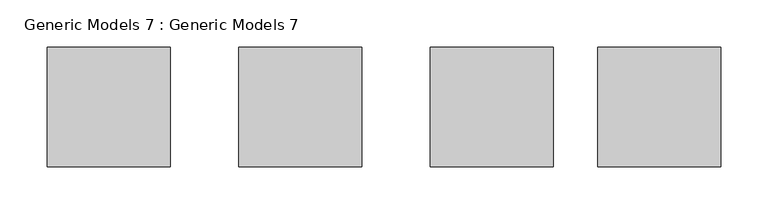
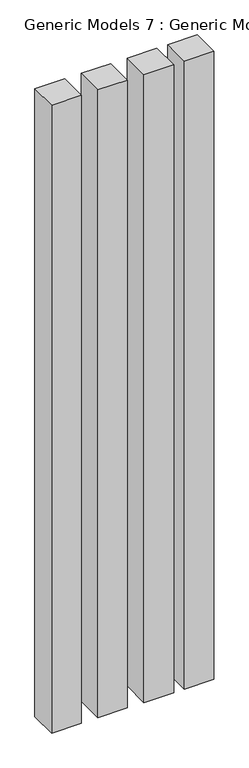
"""IFC4 building model written with IfcOpenShell, lengths in millimetres: proxy geometry, Generic Models 7 : Generic Models 7."""

from ifc_helpers import new_model, si_unit, frame, origin, place, context, project, spatial, polyline, outline, extrude, source, transform, mapped, element, save


def generic_models_7_generic_models_7_fd49988f(model_context):
    return source(origin(), model_context, "Body", "SweptSolid", [
        extrude(outline(polyline([(-1402.2058817, -4217.1262081), (-1532.5624971, -4217.1262081), (-1532.5624971, -4090.1262081), (-1402.2058817, -4090.1262081), (-1402.2058817, -4217.1262081)])), frame((0.0, 0.0, 3352.8), z_axis=(0.0, 0.0, 1.0), x_axis=(1.0, 0.0, 0.0)), (0.0, 0.0, 1.0), 2921.9181383),
        extrude(outline(polyline([(-1199.0058817, -4217.1262081), (-1329.3624971, -4217.1262081), (-1329.3624971, -4090.1262081), (-1199.0058817, -4090.1262081), (-1199.0058817, -4217.1262081)])), frame((0.0, 0.0, 3352.8), z_axis=(0.0, 0.0, 1.0), x_axis=(1.0, 0.0, 0.0)), (0.0, 0.0, 1.0), 2921.9181383),
        extrude(outline(polyline([(-995.8058817, -4217.1262081), (-1126.1624971, -4217.1262081), (-1126.1624971, -4090.1262081), (-995.8058817, -4090.1262081), (-995.8058817, -4217.1262081)])), frame((0.0, 0.0, 3352.8), z_axis=(0.0, 0.0, 1.0), x_axis=(1.0, 0.0, 0.0)), (0.0, 0.0, 1.0), 2921.9181383),
        extrude(outline(polyline([(-818.0058817, -4217.1262081), (-948.3624971, -4217.1262081), (-948.3624971, -4090.1262081), (-818.0058817, -4090.1262081), (-818.0058817, -4217.1262081)])), frame((0.0, 0.0, 3352.8), z_axis=(0.0, 0.0, 1.0), x_axis=(1.0, 0.0, 0.0)), (0.0, 0.0, 1.0), 2921.9181383),
    ])


if __name__ == "__main__":
    model = new_model("IFC4")
    model_context = context("Model", 3, world=origin())
    ifc_project = project(units=[si_unit("LENGTHUNIT", "METRE", prefix="MILLI")], contexts=[model_context])
    site = spatial("IfcSite", under=ifc_project)
    building = spatial("IfcBuilding", under=site)
    placement = place(None, origin())
    generic_models_7_generic_models_7_shape = generic_models_7_generic_models_7_fd49988f(model_context)
    element("IfcBuildingElementProxy", 1, Name="Generic Models 7 : Generic Models 7", ObjectType="Generic Models 7 : Generic Models 7", at=placement, inside=building, context=model_context, shape_type="MappedRepresentation", body=[
        mapped(generic_models_7_generic_models_7_shape, transform((0.0, 0.0, 0.0), x_axis=(1.0, 0.0, 0.0), y_axis=(0.0, 1.0, 0.0), z_axis=(0.0, 0.0, 1.0))),
    ])
    save(model, "model.ifc")
